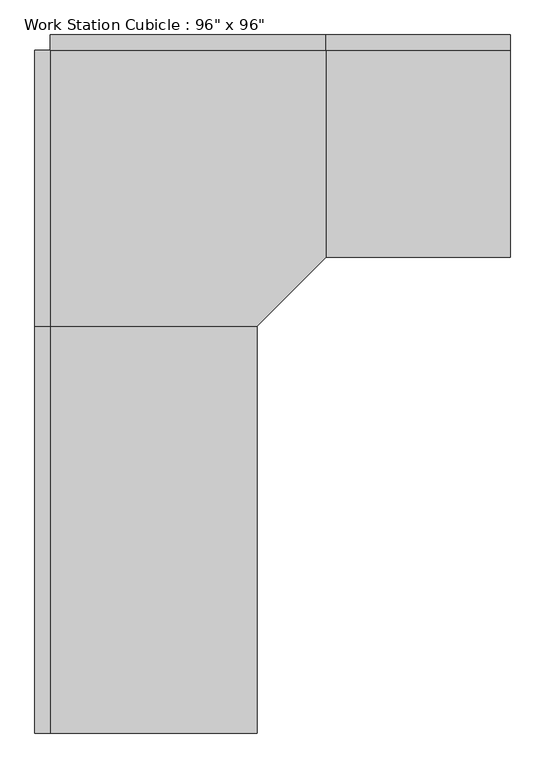
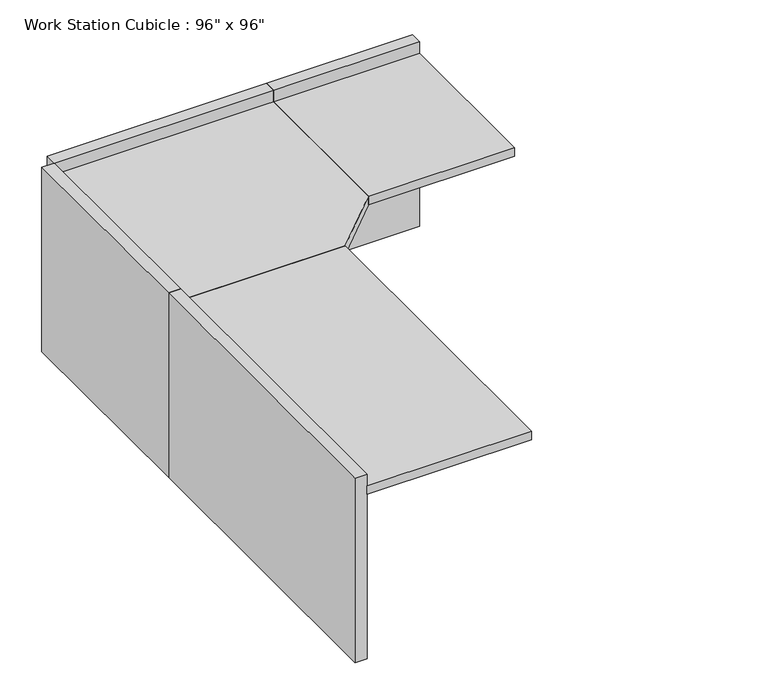
"""IFC4 building model written with IfcOpenShell, lengths in millimetres: furniture geometry."""

from ifc_helpers import new_model, si_unit, frame, origin, origin_with_axes, place, context, project, spatial, polyline, outline, extrude, source, transform, mapped, element, save


def furniture_b52c1e80(model_context):
    return source(origin(), model_context, "Body", "SweptSolid", [
        extrude(outline(polyline([(-80.9317522, -545.8230076), (833.4682478, -545.8230076), (833.4682478, -1231.6230076), (604.8682478, -1460.2230076), (-80.9317522, -1460.2230076), (-80.9317522, -545.8230076)])), frame((0.0, 0.0, 723.9), z_axis=(0.0, 0.0, 1.0), x_axis=(1.0, 0.0, 0.0)), (0.0, 0.0, 1.0), 38.1),
        extrude(outline(polyline([(604.8682478, -2806.4230076), (-80.9317522, -2806.4230076), (-80.9317522, -1460.2230076), (604.8682478, -1460.2230076), (604.8682478, -2806.4230076)])), frame((0.0, 0.0, 723.9), z_axis=(0.0, 0.0, 1.0), x_axis=(1.0, 0.0, 0.0)), (0.0, 0.0, 1.0), 38.1),
        extrude(outline(polyline([(1443.0682478, -1231.6230076), (833.4682478, -1231.6230076), (833.4682478, -545.8230076), (1443.0682478, -545.8230076), (1443.0682478, -1231.6230076)])), frame((0.0, 0.0, 723.9), z_axis=(0.0, 0.0, 1.0), x_axis=(1.0, 0.0, 0.0)), (0.0, 0.0, 1.0), 38.1),
        extrude(outline(polyline([(1443.0682478, -545.8230076), (833.4682478, -545.8230076), (833.4682478, -495.0230076), (1443.0682478, -495.0230076), (1443.0682478, -545.8230076)])), origin_with_axes(), (0.0, 0.0, 1.0), 812.8),
        extrude(outline(polyline([(833.4682478, -545.8230076), (-80.9317522, -545.8230076), (-80.9317522, -495.0230076), (833.4682478, -495.0230076), (833.4682478, -545.8230076)])), origin_with_axes(), (0.0, 0.0, 1.0), 812.8),
        extrude(outline(polyline([(-80.9317522, -1460.2230076), (-131.7317522, -1460.2230076), (-131.7317522, -545.8230076), (-80.9317522, -545.8230076), (-80.9317522, -1460.2230076)])), origin_with_axes(), (0.0, 0.0, 1.0), 812.8),
        extrude(outline(polyline([(-80.9317522, -2806.4230076), (-131.7317522, -2806.4230076), (-131.7317522, -1460.2230076), (-80.9317522, -1460.2230076), (-80.9317522, -2806.4230076)])), origin_with_axes(), (0.0, 0.0, 1.0), 812.8),
    ])


if __name__ == "__main__":
    model = new_model("IFC4")
    model_context = context("Model", 3, world=origin())
    ifc_project = project(units=[si_unit("LENGTHUNIT", "METRE", prefix="MILLI")], contexts=[model_context])
    site = spatial("IfcSite", under=ifc_project)
    building = spatial("IfcBuilding", under=site)
    placement = place(None, origin())
    furniture_shape = furniture_b52c1e80(model_context)
    element("IfcFurniture", 1, ObjectType="Work Station Cubicle : 96\" x 96\"", at=placement, inside=building, context=model_context, shape_type="MappedRepresentation", body=[
        mapped(furniture_shape, transform((0.0, 0.0, 0.0), x_axis=(1.0, 0.0, 0.0), y_axis=(0.0, 1.0, 0.0), z_axis=(0.0, 0.0, 1.0))),
    ])
    save(model, "model.ifc")

# Revit data of these elements
# Type "Work Station Cubicle : 96\" x 96\""
#   Assembly Code = "E2020"
#   Desktop Height = 2' - 6"
#   Desktop1 Width = 2' - 3"
#   Desktop2 Width = 2' - 3"
#   Panel Height = 2' - 8"
#   Panel1 Length = 4' - 5"
#   Panel2 Length = 2' - 0"
#   Cube Panel Material = Textile - Light Gray
#   Work Top Material = Laminate, Ivory, Matte
#   Default Elevation = 0
# Element 1 (IfcFurniture, "Work Station Cubicle : 96\" x 96\"")
#   Materials on its faces: "Textile - Light Gray", "Laminate, Ivory, Matte"
# Materials
#   "Textile - Light Gray": class "Fabric", colour RGB 204 204 204, transparency 0
#   "Laminate, Ivory, Matte": class "Plastic", colour RGB 247 247 239, transparency 0, Description = "Plastic Laminate - Ivory, Matte", Cost = 0
